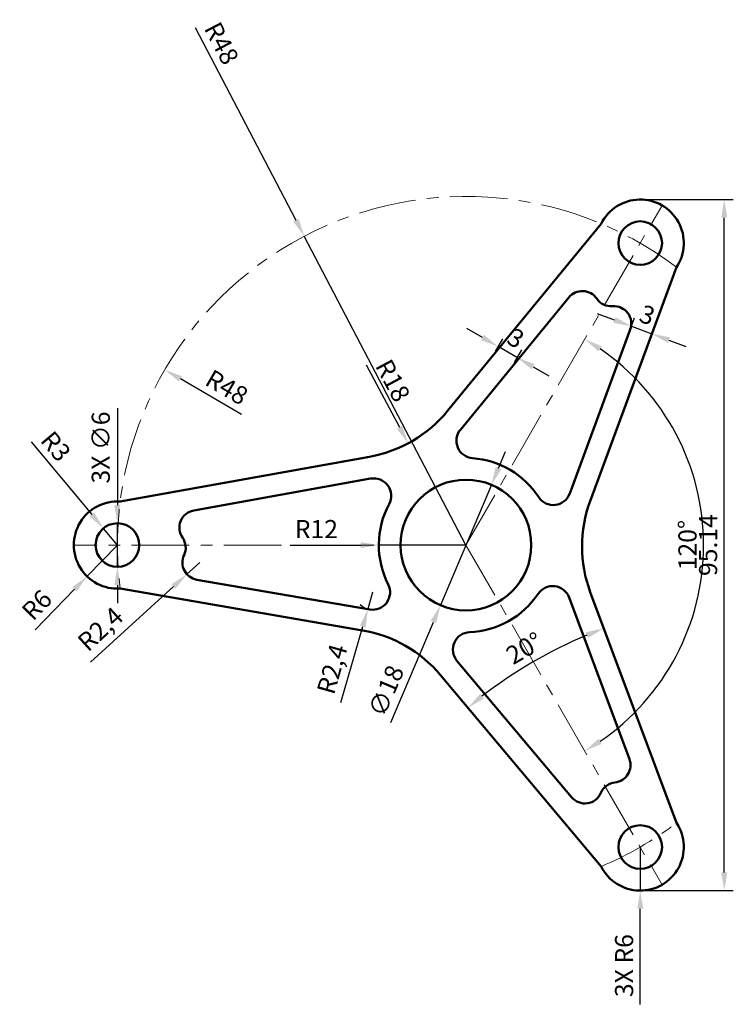
# Model space of a CAD drawing. Units: millimetres. Extents: x 3196 to 3294, y 1250 to 1385.
import ezdxf

# ---------------------------------------------------------------- set-up
doc = ezdxf.new("R2010")
doc.units = ezdxf.units.MM
doc.linetypes.add('CENTER', pattern=[50.8, 31.75, -6.35, 6.35, -6.35])
for name, color, linetype, lineweight in [('M-CNTR', 4, 'CENTER', 18), ('M-DIMS', 2, 'Continuous', 25), ('M-OUTL', 7, 'Continuous', 50)]:
    doc.layers.add(name, color=color, linetype=linetype, lineweight=lineweight)
doc.styles.get("Standard").update_dxf_attribs({"font": 'arial.ttf'})
doc.dimstyles.new('ISO-25', dxfattribs={"dimtxt": 2.5, "dimasz": 2.5, "dimexe": 1.25, "dimexo": 0.625, "dimtad": 1, "dimtxsty": 'Standard', "dimcen": 2.5, "dimadec": 0, "dimazin": 0, "dimtfac": 1, "dimtmove": 0, "dimatfit": 3, "dimfxl": 1, "dimarcsym": 0})

# ---------------------------------------------------------------- blocks, each defined once
blk = doc.blocks.new('*D1')
at = {"layer": 'Defpoints', "color": 0, "transparency": 16777216}
for p in [(3284.55, 1359.56), (3257.55, 1312.79), (3257.55, 1312.79), (3288.3, 1301.6), (3284.55, 1266.03)]:
    blk.add_point(p, dxfattribs=at)
at = {"layer": 'M-DIMS', "color": 0, "lineweight": -2, "transparency": 16777216}
blk.add_arc((3257.55, 1312.79), 32.73, 304.3776, 55.6224, dxfattribs=at)
at = {"layer": 'M-DIMS', "color": 0, "transparency": 16777216}
for points in [[(3275.81, 1339.45), (3276.25, 1340.16), (3273.91, 1341.14)], [(3276.25, 1285.43), (3275.81, 1286.13), (3273.91, 1284.45)]]:
    blk.add_solid(points, dxfattribs=at)
at = {"layer": 'M-DIMS', "color": 0, "transparency": 16777216, "insert": (3288.38, 1312.79), "char_height": 2.5, "attachment_point": 5, "rotation": 90}
blk.add_mtext('120°', dxfattribs=at)
blk = doc.blocks.new('*D2')
at = {"layer": 'Defpoints', "color": 0, "transparency": 16777216}
for p in [(3207.62, 1315.09), (3209.55, 1312.79)]:
    blk.add_point(p, dxfattribs=at)
at = {"layer": 'M-DIMS', "color": 0, "lineweight": -2, "transparency": 16777216}
for p, q in [((3197.66, 1326.99), (3206.02, 1317.01)), ((3209.55, 1312.79), (3207.62, 1315.09))]:
    blk.add_line(p, q, dxfattribs=at)
at = {"layer": 'M-DIMS', "color": 0, "transparency": 16777216}
blk.add_solid([(3206.34, 1317.28), (3205.7, 1316.74), (3207.62, 1315.09)], dxfattribs=at)
at = {"layer": 'M-DIMS', "color": 0, "transparency": 16777216, "insert": (3200.82, 1326.18), "char_height": 2.5, "attachment_point": 5, "rotation": 309.9489}
blk.add_mtext('R3', dxfattribs=at)
blk = doc.blocks.new('*D3')
at = {"layer": 'Defpoints', "color": 0, "transparency": 16777216}
for p in [(3209.55, 1312.79), (3205.37, 1308.49)]:
    blk.add_point(p, dxfattribs=at)
at = {"layer": 'M-DIMS', "color": 0, "lineweight": -2, "transparency": 16777216}
for p, q in [((3209.55, 1312.79), (3205.37, 1308.49)), ((3198.21, 1301.11), (3203.63, 1306.7))]:
    blk.add_line(p, q, dxfattribs=at)
at = {"layer": 'M-DIMS', "color": 0, "transparency": 16777216}
blk.add_solid([(3203.33, 1306.99), (3203.93, 1306.41), (3205.37, 1308.49)], dxfattribs=at)
at = {"layer": 'M-DIMS', "color": 0, "transparency": 16777216, "insert": (3198.68, 1304.33), "char_height": 2.5, "attachment_point": 5, "rotation": 45.8375}
blk.add_mtext('R6', dxfattribs=at)
blk = doc.blocks.new('*D4')
at = {"layer": 'Defpoints', "color": 0, "transparency": 16777216}
for p in [(3220.9, 1310.39), (3219.12, 1308.78)]:
    blk.add_point(p, dxfattribs=at)
at = {"layer": 'M-DIMS', "color": 0, "lineweight": -2, "transparency": 16777216}
for p, q in [((3220.9, 1310.39), (3219.12, 1308.78)), ((3205.83, 1296.67), (3217.27, 1307.09))]:
    blk.add_line(p, q, dxfattribs=at)
at = {"layer": 'M-DIMS', "color": 0, "transparency": 16777216}
blk.add_solid([(3216.99, 1307.4), (3217.55, 1306.79), (3219.12, 1308.78)], dxfattribs=at)
at = {"layer": 'M-DIMS', "color": 0, "transparency": 16777216, "insert": (3207.42, 1301), "char_height": 2.5, "attachment_point": 5, "rotation": 42.3202}
blk.add_mtext('R2,4', dxfattribs=at)
blk = doc.blocks.new('*D5')
at = {"layer": 'Defpoints', "color": 0, "transparency": 16777216}
for p in [(3216.06, 1336.93), (3257.55, 1312.79)]:
    blk.add_point(p, dxfattribs=at)
at = {"layer": 'M-DIMS', "color": 0, "lineweight": -2, "transparency": 16777216}
blk.add_line((3226.63, 1330.78), (3218.22, 1335.67), dxfattribs=at)
at = {"layer": 'M-DIMS', "color": 0, "transparency": 16777216}
blk.add_solid([(3218.43, 1336.03), (3218.01, 1335.31), (3216.06, 1336.93)], dxfattribs=at)
at = {"layer": 'M-DIMS', "color": 0, "transparency": 16777216, "insert": (3224.46, 1334.24), "char_height": 2.5, "attachment_point": 5, "rotation": 329.8096}
blk.add_mtext('R48', dxfattribs=at)
blk = doc.blocks.new('*D6')
at = {"layer": 'Defpoints', "color": 0, "transparency": 16777216}
for p in [(3245.55, 1312.79), (3257.55, 1312.79)]:
    blk.add_point(p, dxfattribs=at)
at = {"layer": 'M-DIMS', "color": 0, "lineweight": -2, "transparency": 16777216}
for p, q in [((3233.35, 1312.79), (3243.05, 1312.79)), ((3257.55, 1312.79), (3245.55, 1312.79))]:
    blk.add_line(p, q, dxfattribs=at)
at = {"layer": 'M-DIMS', "color": 0, "transparency": 16777216}
blk.add_solid([(3243.05, 1313.21), (3243.05, 1312.38), (3245.55, 1312.79)], dxfattribs=at)
at = {"layer": 'M-DIMS', "color": 0, "transparency": 16777216, "insert": (3236.95, 1314.67), "char_height": 2.5, "attachment_point": 5}
blk.add_mtext('R12', dxfattribs=at)
blk = doc.blocks.new('*D7')
at = {"layer": 'Defpoints', "color": 0, "transparency": 16777216}
for p in [(3244.7, 1306.29), (3244.04, 1303.98)]:
    blk.add_point(p, dxfattribs=at)
at = {"layer": 'M-DIMS', "color": 0, "lineweight": -2, "transparency": 16777216}
for p, q in [((3244.7, 1306.29), (3244.04, 1303.98)), ((3240.34, 1291.11), (3243.35, 1301.58))]:
    blk.add_line(p, q, dxfattribs=at)
blk.add_arc((3244.7, 1306.29), 2.4, 224.1348, 260.2199, dxfattribs=at)
at = {"layer": 'M-DIMS', "color": 0, "transparency": 16777216}
blk.add_solid([(3242.95, 1301.7), (3243.75, 1301.47), (3244.04, 1303.98)], dxfattribs=at)
at = {"layer": 'M-DIMS', "color": 0, "transparency": 16777216, "insert": (3239.43, 1295.63), "char_height": 2.5, "attachment_point": 5, "rotation": 73.9763}
blk.add_mtext('R2,4', dxfattribs=at)
blk = doc.blocks.new('*D8')
at = {"layer": 'Defpoints', "color": 0, "transparency": 16777216}
for p in [(3241.1, 1342.68), (3249.58, 1326.8)]:
    blk.add_point(p, dxfattribs=at)
at = {"layer": 'M-DIMS', "color": 0, "lineweight": -2, "transparency": 16777216}
blk.add_line((3243.82, 1337.59), (3248.4, 1329), dxfattribs=at)
at = {"layer": 'M-DIMS', "color": 0, "transparency": 16777216}
blk.add_solid([(3248.77, 1329.2), (3248.04, 1328.81), (3249.58, 1326.8)], dxfattribs=at)
at = {"layer": 'M-DIMS', "color": 0, "transparency": 16777216, "insert": (3247.2, 1335.29), "char_height": 2.5, "attachment_point": 5, "rotation": 298.1014}
blk.add_mtext('R18', dxfattribs=at)
blk = doc.blocks.new('*D9')
at = {"layer": 'Defpoints', "color": 0, "transparency": 16777216}
for p in [(3261.99, 1340.11), (3261.3, 1338.92), (3263.94, 1337.4)]:
    blk.add_point(p, dxfattribs=at)
at = {"layer": 'M-DIMS', "color": 0, "lineweight": -2, "transparency": 16777216}
for p, q in [((3259.83, 1341.36), (3257.66, 1342.61)), ((3261.62, 1339.46), (3262.62, 1341.19)), ((3264.63, 1338.59), (3261.99, 1340.11)), ((3264.25, 1337.94), (3265.25, 1339.67)), ((3266.79, 1337.34), (3268.96, 1336.09))]:
    blk.add_line(p, q, dxfattribs=at)
at = {"layer": 'M-DIMS', "color": 0, "transparency": 16777216}
for points in [[(3260.04, 1341.72), (3259.62, 1341), (3261.99, 1340.11)], [(3267, 1337.7), (3266.58, 1336.98), (3264.63, 1338.59)]]:
    blk.add_solid(points, dxfattribs=at)
at = {"layer": 'M-DIMS', "color": 0, "transparency": 16777216, "insert": (3264.26, 1341), "char_height": 2.5, "attachment_point": 5, "rotation": 330}
blk.add_mtext('3', dxfattribs=at)
blk = doc.blocks.new('*D10')
at = {"layer": 'Defpoints', "color": 0, "transparency": 16777216}
for p in [(3283.16, 1341.87), (3276, 1331.16), (3278.82, 1330.12)]:
    blk.add_point(p, dxfattribs=at)
at = {"layer": 'M-DIMS', "color": 0, "lineweight": -2, "transparency": 16777216}
for p, q in [((3278, 1343.77), (3275.65, 1344.64)), ((3276.22, 1331.75), (3280.78, 1344.08)), ((3279.03, 1330.71), (3283.59, 1343.04)), ((3280.34, 1342.91), (3283.16, 1341.87)), ((3285.5, 1341), (3287.85, 1340.13))]:
    blk.add_line(p, q, dxfattribs=at)
at = {"layer": 'M-DIMS', "color": 0, "transparency": 16777216}
for points in [[(3278.14, 1344.16), (3277.85, 1343.38), (3280.34, 1342.91)], [(3285.65, 1341.39), (3285.36, 1340.61), (3283.16, 1341.87)]]:
    blk.add_solid(points, dxfattribs=at)
at = {"layer": 'M-DIMS', "color": 0, "transparency": 16777216, "insert": (3282.41, 1344.17), "char_height": 2.5, "attachment_point": 5, "rotation": 339.7225}
blk.add_mtext('3', dxfattribs=at)
blk = doc.blocks.new('*D11')
at = {"layer": 'Defpoints', "color": 0, "transparency": 16777216}
for p in [(3274.68, 1306.31), (3269.9, 1298.41), (3254.05, 1294.89), (3286.55, 1274.54), (3276.18, 1268.55)]:
    blk.add_point(p, dxfattribs=at)
at = {"layer": 'M-DIMS', "color": 0, "lineweight": -2, "transparency": 16777216}
blk.add_arc((3298.88, 1241.53), 63.84, 112.7333, 127.7951, dxfattribs=at)
at = {"layer": 'M-DIMS', "color": 0, "transparency": 16777216}
for points in [[(3274.06, 1300.79), (3274.37, 1300.02), (3276.54, 1301.33)], [(3260.02, 1291.65), (3259.5, 1292.3), (3257.82, 1290.4)]]:
    blk.add_solid(points, dxfattribs=at)
at = {"layer": 'M-DIMS', "color": 0, "transparency": 16777216, "insert": (3265.75, 1298.31), "char_height": 2.5, "attachment_point": 5, "rotation": 30.2642}
blk.add_mtext('20°', dxfattribs=at)
blk = doc.blocks.new('*D12')
at = {"layer": 'Defpoints', "color": 0, "transparency": 16777216}
for p in [(3261.06, 1321.08), (3254.04, 1304.51)]:
    blk.add_point(p, dxfattribs=at)
at = {"layer": 'M-DIMS', "color": 0, "lineweight": -2, "transparency": 16777216}
for p, q in [((3262.04, 1323.38), (3263.01, 1325.68)), ((3261.06, 1321.08), (3254.04, 1304.51)), ((3247.19, 1288.36), (3253.06, 1302.2))]:
    blk.add_line(p, q, dxfattribs=at)
at = {"layer": 'M-DIMS', "color": 0, "transparency": 16777216}
for points in [[(3261.65, 1323.54), (3262.42, 1323.22), (3261.06, 1321.08)], [(3252.68, 1302.37), (3253.45, 1302.04), (3254.04, 1304.51)]]:
    blk.add_solid(points, dxfattribs=at)
at = {"layer": 'M-DIMS', "color": 0, "transparency": 16777216, "insert": (3246.85, 1292.6), "char_height": 2.5, "attachment_point": 5, "rotation": 67.0382}
blk.add_mtext('∅18', dxfattribs=at)
blk = doc.blocks.new('MOUNTING-LUG-END-D6')
blk.add_circle((0, 0), 3)
blk.add_arc((0, 0), 6, 86.4167, 273.5833)
blk = doc.blocks.new('*D14')
at = {"layer": 'Defpoints', "color": 0, "transparency": 16777216}
for p in [(3281.42, 1360.36), (3293.12, 1360.36), (3281.42, 1265.23)]:
    blk.add_point(p, dxfattribs=at)
at = {"layer": 'M-DIMS', "color": 0, "lineweight": -2, "transparency": 16777216}
for p, q in [((3282.05, 1360.36), (3294.37, 1360.36)), ((3293.12, 1267.73), (3293.12, 1357.86)), ((3282.05, 1265.23), (3294.37, 1265.23))]:
    blk.add_line(p, q, dxfattribs=at)
at = {"layer": 'M-DIMS', "color": 0, "transparency": 16777216}
for points in [[(3292.7, 1357.86), (3293.54, 1357.86), (3293.12, 1360.36)], [(3292.7, 1267.73), (3293.54, 1267.73), (3293.12, 1265.23)]]:
    blk.add_solid(points, dxfattribs=at)
at = {"layer": 'M-DIMS', "color": 0, "transparency": 16777216, "insert": (3291.22, 1312.79), "char_height": 2.5, "attachment_point": 5, "rotation": 90}
blk.add_mtext('95.14', dxfattribs=at)
blk = doc.blocks.new('*D15')
at = {"layer": 'Defpoints', "color": 0, "transparency": 16777216}
for p in [(3209.55, 1315.79), (3209.55, 1309.79)]:
    blk.add_point(p, dxfattribs=at)
at = {"layer": 'M-DIMS', "color": 0, "lineweight": -2, "transparency": 16777216}
for p, q in [((3209.56, 1331.64), (3209.55, 1318.29)), ((3209.55, 1309.79), (3209.55, 1315.79)), ((3209.55, 1307.29), (3209.55, 1304.79))]:
    blk.add_line(p, q, dxfattribs=at)
at = {"layer": 'M-DIMS', "color": 0, "transparency": 16777216}
for points in [[(3209.13, 1318.29), (3209.97, 1318.29), (3209.55, 1315.79)], [(3209.13, 1307.29), (3209.96, 1307.29), (3209.55, 1309.79)]]:
    blk.add_solid(points, dxfattribs=at)
at = {"layer": 'M-DIMS', "color": 0, "transparency": 16777216, "insert": (3207.58, 1326.22), "char_height": 2.5, "attachment_point": 5, "rotation": 89.9809}
blk.add_mtext('3X ∅6', dxfattribs=at)
blk = doc.blocks.new('*D16')
at = {"layer": 'Defpoints', "color": 0, "transparency": 16777216}
for p in [(3281.55, 1271.22), (3281.55, 1265.22)]:
    blk.add_point(p, dxfattribs=at)
at = {"layer": 'M-DIMS', "color": 0, "lineweight": -2, "transparency": 16777216}
for p, q in [((3281.55, 1271.22), (3281.55, 1265.22)), ((3281.55, 1249.57), (3281.55, 1262.72))]:
    blk.add_line(p, q, dxfattribs=at)
at = {"layer": 'M-DIMS', "color": 0, "transparency": 16777216}
blk.add_solid([(3281.13, 1262.72), (3281.97, 1262.72), (3281.55, 1265.22)], dxfattribs=at)
at = {"layer": 'M-DIMS', "color": 0, "transparency": 16777216, "insert": (3279.65, 1254.9), "char_height": 2.5, "attachment_point": 5, "rotation": 90}
blk.add_mtext('3X R6', dxfattribs=at)
blk = doc.blocks.new('*D17')
at = {"layer": 'Defpoints', "color": 0, "transparency": 16777216}
for p in [(3235.29, 1355.32), (3257.55, 1312.79)]:
    blk.add_point(p, dxfattribs=at)
at = {"layer": 'M-DIMS', "color": 0, "lineweight": -2, "transparency": 16777216}
for p, q in [((3220.26, 1384.04), (3234.13, 1357.54)), ((3257.55, 1312.79), (3235.29, 1355.32))]:
    blk.add_line(p, q, dxfattribs=at)
at = {"layer": 'M-DIMS', "color": 0, "transparency": 16777216}
blk.add_solid([(3234.5, 1357.73), (3233.76, 1357.34), (3235.29, 1355.32)], dxfattribs=at)
at = {"layer": 'M-DIMS', "color": 0, "transparency": 16777216, "insert": (3223.62, 1381.72), "char_height": 2.5, "attachment_point": 5, "rotation": 297.6287}
blk.add_mtext('R48', dxfattribs=at)

msp = doc.modelspace()

# ---------------------------------------------------------------- linework, layer by layer
at = {"layer": 'M-CNTR', "ltscale": 0.25, "transparency": 33554534}
for q in [(3284.549, 1359.559), (3203.549, 1312.793), (3284.549, 1266.028)]:
    msp.add_line((3257.549, 1312.793), q, dxfattribs=at)
for start, end in [(52.83336, 187.16664), (292.83336, 307.16664)]:
    msp.add_arc((3257.549, 1312.793), 48, start, end, dxfattribs=at)
at = {"layer": 'M-OUTL'}
for p, q in [((3276.176, 1357.032), (3255.015, 1331.255)), ((3286.547, 1351.044), (3274.653, 1318.851)), ((3271.724, 1346.882), (3256.779, 1328.675)), ((3280.175, 1342.451), (3271.833, 1319.873)), ((3209.924, 1318.782), (3244.288, 1324.96)), ((3220.057, 1317.556), (3244.421, 1321.936)), ((3220.489, 1308.028), (3244.293, 1303.925)), ((3209.924, 1306.805), (3243.325, 1301.048)), ((3280.056, 1283.343), (3271.743, 1305.592)), ((3286.547, 1274.543), (3274.676, 1306.312)), ((3272.091, 1278.079), (3256.309, 1296.862)), ((3276.176, 1268.555), (3254.048, 1294.889))]:
    msp.add_line(p, q, dxfattribs=at)
msp.add_circle((3257.549, 1312.793), 9, dxfattribs=at)
for centre, radius, start, end in [((3273.579, 1345.359), 2.4, 34.35389, 140.61712), ((3277.542, 1348.068), 2.4, 214.35389, 274.55442), ((3277.923, 1343.283), 2.4, 339.72247, 94.55442), ((3241.103, 1342.676), 18, 280.19292, 320.61712), ((3258.634, 1327.153), 2.4, 140.61712, 265.68034), ((3257.549, 1312.793), 12, 33.32373, 85.68034), ((3244.845, 1319.574), 2.4, 331.90909, 100.19292), ((3269.581, 1320.704), 2.4, 213.32373, 339.72247), ((3291.538, 1312.612), 18, 159.72247, 200.48935), ((3220.482, 1315.193), 2.4, 100.19292, 215.06052), ((3257.549, 1312.793), 12, 151.90909, 206.8473), ((3216.553, 1312.436), 2.4, 334.81397, 35.06052), ((3220.897, 1310.393), 2.4, 154.81397, 260.2199), ((3244.701, 1306.29), 2.4, 260.2199, 26.8473), ((3269.495, 1304.752), 2.4, 20.48935, 146.05271), ((3257.549, 1312.793), 12, 272.37641, 326.05271), ((3240.267, 1283.309), 18, 40.03908, 80.2199), ((3258.146, 1298.406), 2.4, 92.37641, 220.03908), ((3277.808, 1282.503), 2.4, 276.37523, 20.48935), ((3278.341, 1277.733), 2.4, 96.37523, 156.81655), ((3273.929, 1279.623), 2.4, 220.03908, 336.81655)]:
    msp.add_arc(centre, radius, start, end, dxfattribs=at)

# ---------------------------------------------------------------- block references
for p, rotation in [((3281.549, 1354.363), 239.9999999999581), ((3281.549, 1271.224), 119.9999999999566)]:
    msp.add_blockref('MOUNTING-LUG-END-D6', p, dxfattribs=dict(at, rotation=rotation))
msp.add_blockref('MOUNTING-LUG-END-D6', (3209.549, 1312.793), dxfattribs=at)

# ---------------------------------------------------------------- dimensions: what is measured, and where the dimension line sits
at = {"layer": 'M-DIMS'}
for center, mpoint, override, picture, middle in [((3257.549, 1312.793), (3235.289, 1355.32), {"dimdec": 0, "dimlfac": 1, "dimrnd": 0, "dimzin": 0, "dimdsep": 46, "dimlunit": 2}, '*D17', (3221.934, 1380.836)), ((3241.103, 1342.676), (3249.581, 1326.798), {"dimclrd": 0, "dimclre": 0, "dimclrt": 0}, '*D8', (3245.523, 1334.397)), ((3257.549, 1312.793), (3216.06, 1336.931), {"dimclrd": 0, "dimclre": 0, "dimclrt": 0}, '*D5', (3223.506, 1332.599)), ((3209.549, 1312.793), (3207.623, 1315.093), {"dimclrd": 0, "dimclre": 0, "dimclrt": 0}, '*D2', (3199.357, 1324.962)), ((3220.897, 1310.393), (3219.122, 1308.778), {"dimclrd": 0, "dimclre": 0, "dimclrt": 0}, '*D4', (3208.851, 1299.425)), ((3244.701, 1306.29), (3244.039, 1303.983), {"dimclrd": 0, "dimclre": 0, "dimclrt": 0}, '*D7', (3241.472, 1295.047))]:
    dim = msp.add_radius_dim(center=center, mpoint=mpoint, dimstyle='ISO-25', override=override, dxfattribs=at)
    dim.commit()
    dim.dimension.update_dxf_attribs({"geometry": picture, "text_midpoint": middle, "dimtype": 164})
for base, line1, line2, picture, middle in [((3288.304, 1301.6), ((3257.549, 1312.793), (3284.549, 1359.559)), ((3257.549, 1312.793), (3284.549, 1266.028)), '*D1', (3288.376, 1312.793)), ((3269.897, 1298.406), ((3286.547, 1274.543), (3274.676, 1306.312)), ((3276.176, 1268.555), (3254.048, 1294.889)), '*D11', (3265.753, 1298.308))]:
    dim = msp.add_angular_dim_2l(base=base, line1=line1, line2=line2, dimstyle='ISO-25', override={"dimclrd": 0, "dimclre": 0, "dimclrt": 0}, dxfattribs=at)
    dim.commit()
    dim.dimension.update_dxf_attribs({"geometry": picture, "text_midpoint": middle})
dim = msp.add_linear_dim(base=(3293.1188, 1360.3614), p1=(3281.4239, 1265.2255), p2=(3281.4239, 1360.3614), angle=90, dimstyle='ISO-25', override={"dimdec": 2, "dimlfac": 1, "dimrnd": 0, "dimzin": 0, "dimdsep": 46, "dimlunit": 2}, dxfattribs=at)
dim.commit()
dim.dimension.update_dxf_attribs({"geometry": '*D14', "text_midpoint": (3291.2174, 1312.7935)})
for p1, p2, distance, override, picture, middle in [((3276.004, 1331.162), (3278.818, 1330.122), 12.519, {"dimclrd": 0, "dimclre": 0, "dimclrt": 0}, '*D10', (3282.409, 1344.17)), ((3263.937, 1337.395), (3261.304, 1338.916), -1.38, {"dimdec": 0, "dimclrd": 0, "dimclre": 0, "dimclrt": 0}, '*D9', (3264.262, 1340.998))]:
    dim = msp.add_aligned_dim(p1=p1, p2=p2, distance=distance, dimstyle='ISO-25', override=override, dxfattribs=at)
    dim.commit()
    dim.dimension.update_dxf_attribs({"geometry": picture, "text_midpoint": middle})
dim = msp.add_diameter_dim_2p(p1=(3209.548, 1309.793), p2=(3209.55, 1315.793), text='3X <>', dimstyle='ISO-25', override={"dimdec": 0, "dimlfac": 1, "dimrnd": 0, "dimzin": 0, "dimdsep": 46, "dimlunit": 2}, dxfattribs=at)
dim.commit()
dim.dimension.update_dxf_attribs({"geometry": '*D15', "text_midpoint": (3209.553, 1326.216)})
dim = msp.add_diameter_dim_2p(p1=(3261.06, 1321.08), p2=(3254.038, 1304.507), dimstyle='ISO-25', override={"dimclrd": 0, "dimclre": 0, "dimclrt": 0}, dxfattribs=at)
dim.commit()
dim.dimension.update_dxf_attribs({"geometry": '*D12', "text_midpoint": (3248.669, 1291.834), "dimtype": 163})
for center, mpoint, picture, middle in [((3257.549, 1312.793), (3245.549, 1312.793), '*D6', (3236.95, 1314.674)), ((3209.549, 1312.793), (3205.369, 1308.489), '*D3', (3198.682, 1304.333))]:
    dim = msp.add_radius_dim(center=center, mpoint=mpoint, dimstyle='ISO-25', override={"dimclrd": 0, "dimclre": 0, "dimclrt": 0}, dxfattribs=at)
    dim.commit()
    dim.dimension.update_dxf_attribs({"geometry": picture, "text_midpoint": middle})
dim = msp.add_radius_dim(center=(3281.549, 1271.224), mpoint=(3281.549, 1265.224), text='3X <>', dimstyle='ISO-25', override={"dimdec": 0, "dimlfac": 1, "dimrnd": 0, "dimzin": 0, "dimdsep": 46, "dimlunit": 2}, dxfattribs=at)
dim.commit()
dim.dimension.update_dxf_attribs({"geometry": '*D16', "text_midpoint": (3279.647, 1254.899)})

doc.saveas('drawing.dxf')
